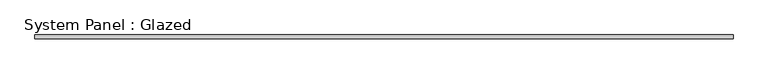
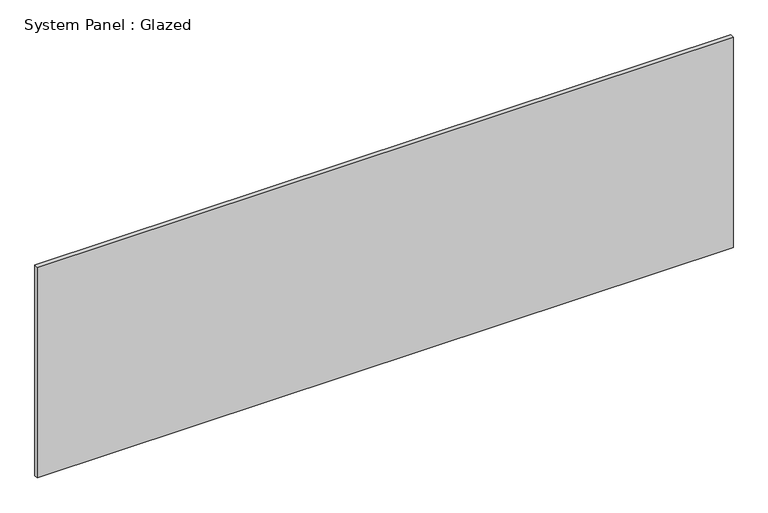
"""IFC4 building model written with IfcOpenShell, lengths in millimetres: plate geometry, System Panel : Glazed."""

from ifc_helpers import new_model, si_unit, origin, origin_with_axes, place, context, project, spatial, polyline, outline, extrude, source, transform, mapped, element, save


def system_panel_glazed_3a6cb6e4(model_context):
    return source(origin(), model_context, "Body", "SweptSolid", [
        extrude(outline(polyline([(2282.2183756, 19.05), (-2282.2183756, 19.05), (-2282.2183756, 44.45), (2282.2183756, 44.45), (2282.2183756, 19.05)])), origin_with_axes(), (0.0, 0.0, 1.0), 1460.5),
    ])


if __name__ == "__main__":
    model = new_model("IFC4")
    model_context = context("Model", 3, world=origin())
    ifc_project = project(units=[si_unit("LENGTHUNIT", "METRE", prefix="MILLI")], contexts=[model_context])
    site = spatial("IfcSite", under=ifc_project)
    building = spatial("IfcBuilding", under=site)
    placement = place(None, origin())
    system_panel_glazed_shape = system_panel_glazed_3a6cb6e4(model_context)
    element("IfcPlate", 1, ObjectType="System Panel : Glazed", at=placement, inside=building, context=model_context, shape_type="MappedRepresentation", body=[
        mapped(system_panel_glazed_shape, transform((0.0, 0.0, 0.0), x_axis=(1.0, 0.0, 0.0), y_axis=(0.0, 1.0, 0.0), z_axis=(0.0, 0.0, 1.0))),
    ])
    save(model, "model.ifc")

# Revit data of these elements
# Type "System Panel : Glazed"
#   Construction Type Id = "GSP4R"
#   Analytic Construction = "1/8 in Pilkington single glazing"
#   Visual Light Transmittance = 0.9
#   Solar Heat Gain Coefficient = 0.86
#   Heat Transfer Coefficient (U) = 1.18115 BTU/(h·ft²·°F)
# Element 1 (IfcPlate, "System Panel : Glazed")
#   Materials on its faces: "Glass"
# Materials
#   "Glass": class "Glass", colour RGB 0 128 192, transparency 0.75, Description = "Soda Lime Glass", Cost = 0
